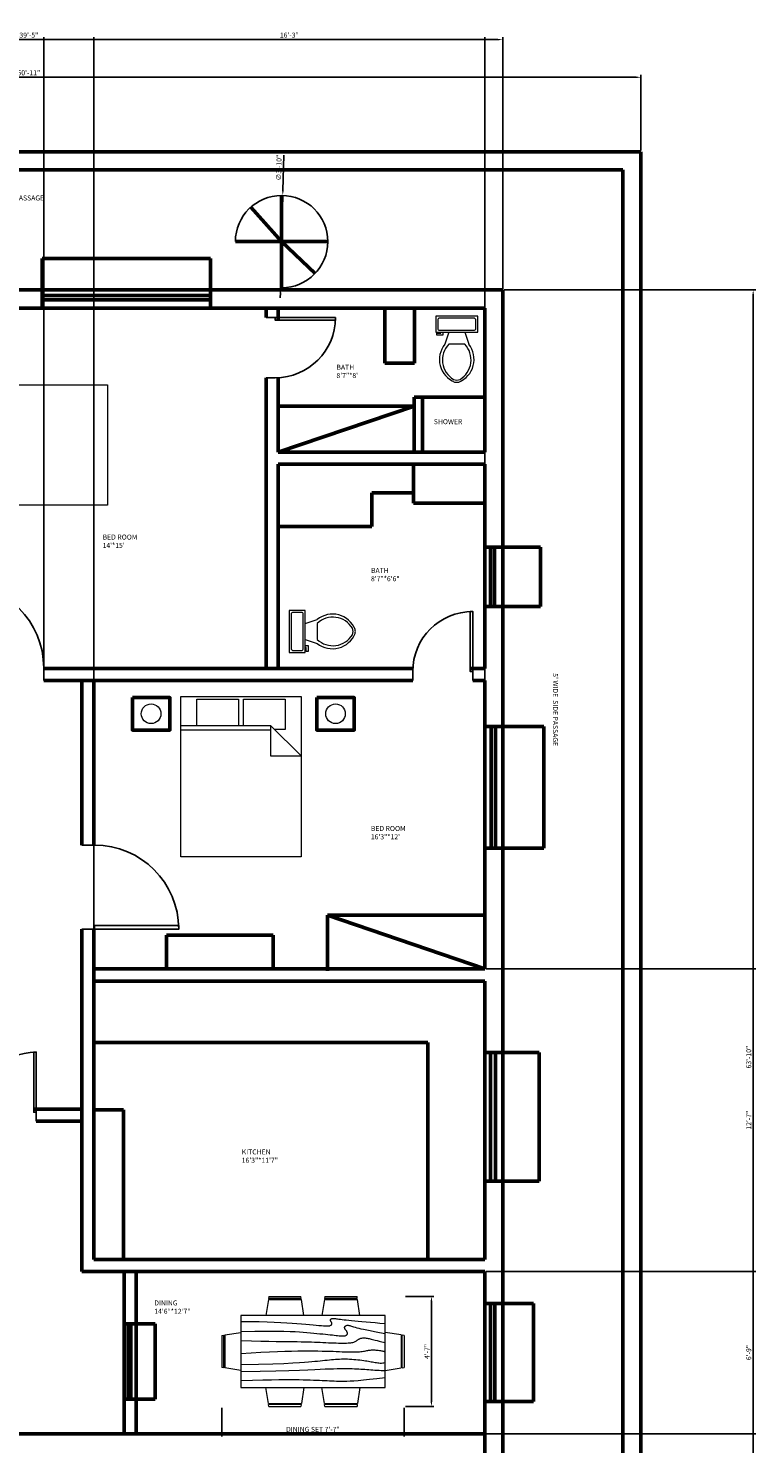
# Model space of a CAD drawing. Units: inches. Extents: x 5312 to 23584, y 2846 to 7447.
# Tile 11 of 12: x 11753 to 12116, y 3367 to 4074. Entities that reach past the tile are written whole.
import ezdxf

# ---------------------------------------------------------------- set-up
doc = ezdxf.new("R2010")
doc.units = ezdxf.units.IN
for name, color, linetype, lineweight in [('A-ANNO-DIMS', 2, 'Continuous', 18), ('A-ANNO-TEXT', 3, 'Continuous', 18), ('A-AREA-IDEN', 7, 'Continuous', 18), ('A-DOOR', 4, 'Continuous', 25), ('A-FLOR-FIXT', 9, 'Continuous', 18), ('A-FURN', 8, 'Continuous', 18), ('A-WALL', 7, 'Continuous', 50)]:
    doc.layers.add(name, color=color, linetype=linetype, lineweight=lineweight)
doc.styles.get("Standard").update_dxf_attribs({"font": 'arial.ttf'})
doc.dimstyles.new('ISO-25', dxfattribs={"dimtxt": 2.5, "dimasz": 2.5, "dimexe": 1.25, "dimexo": 0.625, "dimtad": 1, "dimlunit": 3, "dimtxsty": 'Standard', "dimcen": 2.5, "dimadec": 0, "dimazin": 0, "dimtfac": 1, "dimtmove": 0, "dimatfit": 3, "dimfxl": 1, "dimarcsym": 0})

# ---------------------------------------------------------------- blocks, each defined once
blk = doc.blocks.new('*U2')
for p, q in [((0, 0), (0, -6)), ((40, 0), (40, -6))]:
    blk.add_line(p, q)
blk.add_lwpolyline([(0, 0), (0, 40), (1.75, 40), (1.75, 0)], close=True)
blk.add_arc((0, 0), 40, 0, 90)
blk = doc.blocks.new('Toilet - top')
for p, q in [((9.5, -6), (9.5, -2)), ((-10, -8.5), (-8, -8.5)), ((-10, -9.5), (-10, -8.5)), ((-7, -9.5), (-10, -9.5)), ((-8, -8.5), (-8, -8)), ((-7, -8), (-7, -9.5)), ((-4, -8), (-6, -14)), ((4, -14), (-4, -14)), ((4, -8), (6, -14))]:
    blk.add_line(p, q)
blk.add_lwpolyline([(10.5, -8), (10.5, 0), (-10.5, 0), (-10.5, -8)], close=True)
for points in [[(-9.5, -2), (-9.5, -6)], [(8.5, -1), (-8.5, -1)], [(-8.5, -7), (8.5, -7)]]:
    blk.add_lwpolyline(points)
for centre, radius, start, end in [((-8.62, -1.88), 0.884, 81.8699, 188.1301), ((-8.62, -6.12), 0.884, 171.8699, 278.1301), ((8.62, -1.88), 0.884, 351.8699, 98.1301), ((8.62, -6.12), 0.884, 261.8699, 8.1301), ((3.52, -21.58), 12.17, 141.46911, 247.97143), ((4.2, -21.82), 11.33, 136.36773, 238.94682), ((-3.52, -21.58), 12.17, 292.02843, 38.53071), ((-4.2, -21.82), 11.33, 301.05301, 43.63209), ((0, -27.88), 4, 245.73182, 294.26817), ((0, -29), 4, 254.86053, 285.13947)]:
    blk.add_arc(centre, radius, start, end)
blk = doc.blocks.new('Bed - Queen')
for p, q in [((0, -80.00003), (0, 0)), ((0, 0), (59.99999, 0)), ((59.99999, 0), (59.99999, -80.00003)), ((7.99999, -1.2), (28.79998, -1.2)), ((7.99999, -14.4), (7.99999, -1.2)), ((28.79998, -1.2), (28.79998, -14.4)), ((31.19999, -1.2), (51.99999, -1.2)), ((31.19999, -14.4), (31.19999, -1.2)), ((51.99999, -1.2), (51.99999, -16.4)), ((0, -14.4), (44.8, -14.4)), ((44.8, -16.8), (0, -16.8)), ((59.99999, -29.6), (44.8, -14.4)), ((44.8, -14.4), (44.8, -29.6)), ((51.99999, -16.4), (46.79936, -16.4)), ((44.8, -29.6), (59.99999, -29.6)), ((59.99999, -80.00003), (0, -80.00003))]:
    blk.add_line(p, q)
blk = doc.blocks.new('Dining Set - 36 x 72 in.')
for p, q in [((-22.2343, 26.00059), (-23.4847, 17.99762)), ((-22.2304, 26), (-5.7608, 26)), ((-22, 27.5), (-22.1562, 26.50042)), ((-5.8416, 26.5), (-22.1534, 26.5)), ((-22, 27.5), (-6, 27.5)), ((-5.8437, 26.49966), (-6, 27.5)), ((-4.5152, 17.99762), (-5.7655, 25.99926)), ((5.7657, 26.00059), (4.5153, 17.99762)), ((5.7696, 26), (22.2392, 26)), ((6, 27.5), (5.8438, 26.50042)), ((22.1584, 26.5), (5.8466, 26.5)), ((6, 27.5), (22, 27.5)), ((22.1563, 26.49966), (22, 27.5)), ((23.4848, 17.99762), (22.2345, 25.99926)), ((36, 18), (-36, 18)), ((-36, 18), (-36, -18)), ((36, -18), (36, 18)), ((-45.5, 8), (-44.5004, 8.15617)), ((-45.5, 8), (-45.5, -8)), ((-44.5, -8.15843), (-44.5, 8.15338)), ((-44.0006, 8.23428), (-35.9976, 9.48474)), ((-44, 8.23041), (-44, -8.23915)), ((44.0006, 8.23428), (35.9976, 9.48474)), ((44, 8.23041), (44, -8.23915)), ((44.5, -8.15843), (44.5, 8.15338)), ((45.5, 8), (44.5005, 8.15617)), ((45.5, 8), (45.5, -8)), ((-44.4997, -8.15631), (-45.5, -8)), ((-35.9976, -9.48476), (-43.9993, -8.2345)), ((35.9976, -9.48476), (43.9993, -8.2345)), ((44.4997, -8.15631), (45.5, -8)), ((-36, -18), (36, -18)), ((-22.2343, -26.0006), (-23.4847, -17.99762)), ((-4.5152, -17.99762), (-5.7655, -25.99928)), ((5.7657, -26.0006), (4.5153, -17.99762)), ((23.4848, -17.99762), (22.2345, -25.99928)), ((-22.2304, -26), (-5.7608, -26)), ((-22, -27.5), (-22.1562, -26.50044)), ((-5.8416, -26.5), (-22.1534, -26.5)), ((-22, -27.5), (-6, -27.5)), ((-5.8437, -26.49967), (-6, -27.5)), ((5.7696, -26), (22.2392, -26)), ((6, -27.5), (5.8438, -26.50044)), ((22.1584, -26.5), (5.8466, -26.5)), ((6, -27.5), (22, -27.5)), ((22.1563, -26.49967), (22, -27.5))]:
    blk.add_line(p, q)
for points in [[(-36, 15), (-31.1772, 14.97754), (-26.8079, 14.91406), (-22.8538, 14.81543), (-19.276, 14.6875), (-16.0362, 14.53613), (-13.0957, 14.36718), (-10.4159, 14.18652), (-7.9583, 14), (-5.6904, 13.81315), (-3.6035, 13.63021), (-1.6954, 13.45508), (0.0365, 13.29166), (1.5945, 13.14388), (2.9811, 13.01562), (4.1988, 12.9108), (5.25, 12.83333), (6.1393, 12.78613), (6.8802, 12.76823), (7.4883, 12.77767), (7.9792, 12.8125), (8.3685, 12.87077), (8.6719, 12.95052), (8.9049, 13.0498), (9.0833, 13.16666), (9.2205, 13.29899), (9.3216, 13.44401), (9.3895, 13.59879), (9.4271, 13.76041), (9.4373, 13.92594), (9.4232, 14.09245), (9.3875, 14.257), (9.3333, 14.41666), (9.2638, 14.56917), (9.1836, 14.71484), (9.0975, 14.85465), (9.0104, 14.98958), (8.9272, 15.1206), (8.8529, 15.2487), (8.7922, 15.37483), (8.75, 15.5), (8.7305, 15.62467), (8.7344, 15.74739), (8.7617, 15.86621), (8.8125, 15.97916), (8.8867, 16.08431), (8.9844, 16.17968), (9.1055, 16.26334), (9.25, 16.33333), (9.4189, 16.38802), (9.6172, 16.42708), (9.8506, 16.45052), (10.125, 16.45833), (10.4463, 16.45052), (10.8203, 16.42708), (11.2529, 16.38802), (11.75, 16.33333), (12.3184, 16.26318), (12.9694, 16.17838), (13.7151, 16.07991), (14.5677, 15.96875), (15.5395, 15.84586), (16.6426, 15.71224), (17.8893, 15.56884), (19.2917, 15.41666), (20.859, 15.25667), (22.5879, 15.08984), (24.4721, 14.91715), (26.5052, 14.73958), (28.6809, 14.5581), (30.9929, 14.3737), (33.4347, 14.18733), (36, 14)], [(-36, 10), (-28.9766, 10.14274), (-23.1725, 10.20442), (-18.4241, 10.19775), (-14.5677, 10.13541), (-11.4399, 10.03011), (-8.877, 9.89453), (-6.7154, 9.74137), (-4.7917, 9.58333), (-2.9698, 9.43082), (-1.2246, 9.28515), (0.4415, 9.14534), (2.026, 9.01041), (3.5266, 8.87939), (4.9408, 8.7513), (6.266, 8.62516), (7.5, 8.5), (8.6411, 8.37549), (9.6914, 8.2539), (10.6538, 8.13818), (11.5312, 8.03125), (12.3267, 7.93603), (13.043, 7.85547), (13.6831, 7.79248), (14.25, 7.75), (14.7471, 7.7303), (15.1797, 7.73307), (15.5537, 7.75732), (15.875, 7.80208), (16.1494, 7.86637), (16.3828, 7.94922), (16.5811, 8.04964), (16.75, 8.16666), (16.8944, 8.29915), (17.0143, 8.44531), (17.1089, 8.60319), (17.1771, 8.77083), (17.218, 8.94629), (17.2305, 9.1276), (17.2137, 9.31282), (17.1667, 9.5), (17.0895, 9.6875), (16.987, 9.875), (16.8649, 10.0625), (16.7292, 10.25), (16.5856, 10.4375), (16.4401, 10.625), (16.2985, 10.8125), (16.1667, 11), (16.05, 11.18733), (15.9518, 11.3737), (15.8752, 11.5581), (15.8229, 11.73958), (15.798, 11.91715), (15.8034, 12.08984), (15.842, 12.25667), (15.9167, 12.41666), (16.0295, 12.56836), (16.1784, 12.70833), (16.3605, 12.83268), (16.5729, 12.9375), (16.8127, 13.01888), (17.0768, 13.07291), (17.3625, 13.0957), (17.6667, 13.08333), (17.9894, 13.03312), (18.3418, 12.94726), (18.7382, 12.82918), (19.1927, 12.68229), (19.7195, 12.51001), (20.3327, 12.31575), (21.0465, 12.10294), (21.875, 11.875), (22.8357, 11.63354), (23.959, 11.37304), (25.2786, 11.08618), (26.8282, 10.76562), (28.6414, 10.40405), (30.752, 9.99414), (33.1936, 9.52856), (36, 9)], [(-36, 5.5), (-30.7157, 5.3348), (-26.069, 5.20963), (-21.9946, 5.11767), (-18.4271, 5.05208), (-15.3009, 5.00602), (-12.5508, 4.97265), (-10.1112, 4.94515), (-7.9167, 4.91666), (-5.909, 4.88167), (-4.0586, 4.83984), (-2.3429, 4.79215), (-0.7396, 4.73958), (0.7739, 4.6831), (2.22, 4.6237), (3.6213, 4.56233), (5, 4.5), (6.373, 4.43782), (7.7344, 4.3776), (9.0723, 4.32129), (10.375, 4.27083), (11.6309, 4.22819), (12.8281, 4.19531), (13.9551, 4.17415), (15, 4.16666), (15.954, 4.17448), (16.819, 4.19791), (17.6001, 4.23698), (18.3021, 4.29166), (18.9299, 4.36198), (19.4883, 4.44791), (19.9823, 4.54948), (20.4167, 4.66666), (20.7969, 4.79899), (21.1302, 4.94401), (21.4245, 5.09879), (21.6875, 5.26041), (21.9271, 5.42594), (22.1511, 5.59245), (22.3672, 5.757), (22.5834, 5.91666), (22.8065, 6.06868), (23.0404, 6.21093), (23.2879, 6.34147), (23.5521, 6.45833), (23.8358, 6.55957), (24.142, 6.64323), (24.4735, 6.70735), (24.8334, 6.75), (25.2235, 6.76969), (25.642, 6.76692), (26.0858, 6.74267), (26.5521, 6.69791), (27.0379, 6.63362), (27.5404, 6.55078), (28.0565, 6.45036), (28.5834, 6.33333), (29.1242, 6.19987), (29.7071, 6.04687), (30.3661, 5.87044), (31.1354, 5.66666), (32.0493, 5.43164), (33.142, 5.16146), (34.4475, 4.85221), (36, 4.5)], [(-36, -1), (-30.7915, -0.6591), (-26.0195, -0.38216), (-21.6519, -0.16284), (-17.6563, 0.00521), (-14.0005, 0.12833), (-10.6523, 0.21289), (-7.5796, 0.26522), (-4.75, 0.29166), (-2.134, 0.29793), (0.2878, 0.28711), (2.5317, 0.26163), (4.6146, 0.22396), (6.5529, 0.17651), (8.3633, 0.12174), (10.0623, 0.06209), (11.6667, 0), (13.1899, -0.06201), (14.6341, -0.1211), (15.9982, -0.17432), (17.2813, -0.21875), (18.4823, -0.25147), (19.6003, -0.26953), (20.6343, -0.27002), (21.5834, -0.25), (22.4481, -0.20768), (23.2357, -0.14584), (23.9549, -0.06836), (24.6146, 0.02083), (25.2235, 0.11784), (25.7904, 0.21875), (26.3241, 0.31966), (26.8334, 0.41666), (27.3265, 0.50618), (27.8099, 0.58593), (28.2894, 0.65397), (28.7709, 0.70833), (29.2601, 0.74707), (29.763, 0.76823), (30.2855, 0.76985), (30.8334, 0.75), (31.4088, 0.70784), (31.9994, 0.64713), (32.589, 0.57275), (33.1615, 0.48958), (33.7008, 0.4025), (34.1908, 0.3164), (34.6153, 0.23616), (34.9584, 0.16666), (35.2099, 0.11165), (35.3848, 0.07031), (35.504, 0.04069), (35.5886, 0.02083), (35.6594, 0.00879), (35.7377, 0.0026), (35.8442, 0.00032), (36, 0)], [(-36, -6.5), (-27.1843, -6.31267), (-20.084, -6.1263), (-14.469, -5.9419), (-10.1094, -5.76042), (-6.7752, -5.58285), (-4.2363, -5.41016), (-2.2629, -5.24333), (-0.625, -5.08334), (0.8708, -4.93099), (2.2715, -4.78646), (3.5872, -4.64974), (4.8281, -4.52084), (6.0046, -4.39974), (7.127, -4.28646), (8.2053, -4.18099), (9.25, -4.08334), (10.2705, -3.99382), (11.2734, -3.91407), (12.2647, -3.84603), (13.25, -3.79167), (14.2354, -3.75293), (15.2266, -3.73177), (16.2295, -3.73015), (17.25, -3.75), (18.2912, -3.79248), (19.3451, -3.85547), (20.4009, -3.93604), (21.4479, -4.03125), (22.4754, -4.13819), (23.4727, -4.25391), (24.4289, -4.37549), (25.3334, -4.5), (26.1785, -4.62492), (26.9694, -4.74935), (27.7145, -4.87281), (28.4219, -4.99479), (29.1, -5.11483), (29.7572, -5.23242), (30.4016, -5.34709), (31.0417, -5.45834), (31.6837, -5.56437), (32.3262, -5.65821), (32.9658, -5.73153), (33.599, -5.77604), (34.2224, -5.78345), (34.8327, -5.74545), (35.4264, -5.65373), (36, -5.5)], [(-36, -10), (-26.4022, -9.81299), (-18.4675, -9.62891), (-11.9839, -9.45069), (-6.7396, -9.28125), (-2.5226, -9.12354), (0.8789, -8.98047), (3.6769, -8.85498), (6.0833, -8.75), (8.2767, -8.66765), (10.3021, -8.60677), (12.1712, -8.56543), (13.8958, -8.54167), (15.4876, -8.53353), (16.9583, -8.53907), (18.3197, -8.55632), (19.5834, -8.58334), (20.7616, -8.61841), (21.8685, -8.66081), (22.9188, -8.71004), (23.9271, -8.76563), (24.9081, -8.82707), (25.8763, -8.89388), (26.8465, -8.96558), (27.8334, -9.04167), (28.8474, -9.12118), (29.8828, -9.20117), (30.93, -9.27824), (31.9792, -9.34896), (33.0205, -9.40991), (34.0443, -9.45768), (35.0407, -9.48885), (36, -9.5)], [(-36, -14.5), (-30.0881, -14.33513), (-25.0332, -14.21224), (-20.7312, -14.12647), (-17.0781, -14.07292), (-13.97, -14.04671), (-11.3027, -14.04297), (-8.9724, -14.05681), (-6.875, -14.08334), (-4.9224, -14.11833), (-3.0905, -14.16016), (-1.3709, -14.20785), (0.2448, -14.26042), (1.7647, -14.3169), (3.1973, -14.3763), (4.5507, -14.43767), (5.8333, -14.5), (7.0554, -14.5621), (8.235, -14.62175), (9.3922, -14.67652), (10.5469, -14.72396), (11.7192, -14.76164), (12.929, -14.78711), (14.1965, -14.79794), (15.5417, -14.79167), (16.9933, -14.76424), (18.6152, -14.70508), (20.4804, -14.60197), (22.6615, -14.44271), (25.2312, -14.21509), (28.2624, -13.9069), (31.8277, -13.50594), (36, -13)]]:
    blk.add_lwpolyline(points)
blk = doc.blocks.new('*D19')
at = {"layer": 'A-ANNO-DIMS', "color": 0, "lineweight": -2, "transparency": 16777216}
for p, q in [((11447.29, 4012.53), (11447.29, 4050.35)), ((11449.79, 4049.1), (12055.79, 4049.1)), ((12058.29, 4012.53), (12058.29, 4050.35))]:
    blk.add_line(p, q, dxfattribs=at)
at = {"layer": 'A-ANNO-DIMS', "color": 0, "transparency": 16777216}
for points in [[(11449.79, 4049.52), (11449.79, 4048.69), (11447.29, 4049.1)], [(12055.79, 4049.52), (12055.79, 4048.69), (12058.29, 4049.1)]]:
    blk.add_solid(points, dxfattribs=at)
at = {"layer": 'DEFPOINTS', "color": 0, "transparency": 16777216}
for p in [(12058.29, 4049.1), (11447.29, 4011.91), (12058.29, 4011.91)]:
    blk.add_point(p, dxfattribs=at)
at = {"layer": 'A-ANNO-DIMS', "color": 0, "transparency": 16777216, "insert": (11752.79, 4051.01), "char_height": 2.5, "attachment_point": 5}
blk.add_mtext('50\'-11"', dxfattribs=at)
blk = doc.blocks.new('*D39')
at = {"layer": 'A-ANNO-DIMS', "color": 0, "lineweight": -2, "transparency": 16777216}
for p, q in [((11849.06, 3384.83), (11849.06, 3370.56)), ((11940.06, 3384.83), (11940.06, 3370.56)), ((11851.56, 3371.81), (11937.56, 3371.81))]:
    blk.add_line(p, q, dxfattribs=at)
at = {"layer": 'A-ANNO-DIMS', "color": 0, "transparency": 16777216}
for points in [[(11851.56, 3372.23), (11851.56, 3371.39), (11849.06, 3371.81)], [(11937.56, 3372.23), (11937.56, 3371.39), (11940.06, 3371.81)]]:
    blk.add_solid(points, dxfattribs=at)
at = {"layer": 'DEFPOINTS', "color": 0, "transparency": 16777216}
for p in [(11849.06, 3385.46), (11940.06, 3385.46), (11940.06, 3371.81)]:
    blk.add_point(p, dxfattribs=at)
at = {"layer": 'A-ANNO-DIMS', "color": 0, "transparency": 16777216, "insert": (11894.56, 3373.73), "char_height": 2.5, "attachment_point": 5}
blk.add_mtext('DINING SET 7\'-7"', dxfattribs=at)
blk = doc.blocks.new('*D40')
at = {"layer": 'A-ANNO-DIMS', "color": 0, "lineweight": -2, "transparency": 16777216}
for p, q in [((11940.69, 3440.46), (11954.96, 3440.46)), ((11953.71, 3387.96), (11953.71, 3437.96)), ((11940.69, 3385.46), (11954.96, 3385.46))]:
    blk.add_line(p, q, dxfattribs=at)
at = {"layer": 'A-ANNO-DIMS', "color": 0, "transparency": 16777216}
for points in [[(11953.3, 3437.96), (11954.13, 3437.96), (11953.71, 3440.46)], [(11953.3, 3387.96), (11954.13, 3387.96), (11953.71, 3385.46)]]:
    blk.add_solid(points, dxfattribs=at)
at = {"layer": 'DEFPOINTS', "color": 0, "transparency": 16777216}
for p in [(11940.06, 3440.46), (11953.71, 3440.46), (11940.06, 3385.46)]:
    blk.add_point(p, dxfattribs=at)
at = {"layer": 'A-ANNO-DIMS', "color": 0, "transparency": 16777216, "insert": (11951.84, 3412.96), "char_height": 2.5, "attachment_point": 5, "rotation": 90}
blk.add_mtext('4\'-7"', dxfattribs=at)
blk = doc.blocks.new('*D59')
at = {"layer": 'A-ANNO-DIMS', "color": 0, "lineweight": -2, "transparency": 16777216}
for p, q in [((11516.29, 3943.53), (11516.29, 4069.16)), ((11518.79, 4067.91), (11986.79, 4067.91)), ((11989.29, 3943.53), (11989.29, 4069.16))]:
    blk.add_line(p, q, dxfattribs=at)
at = {"layer": 'A-ANNO-DIMS', "color": 0, "transparency": 16777216}
for points in [[(11518.79, 4068.32), (11518.79, 4067.49), (11516.29, 4067.91)], [(11986.79, 4068.32), (11986.79, 4067.49), (11989.29, 4067.91)]]:
    blk.add_solid(points, dxfattribs=at)
at = {"layer": 'DEFPOINTS', "color": 0, "transparency": 16777216}
for p in [(11989.29, 4067.91), (11516.29, 3942.91), (11989.29, 3942.91)]:
    blk.add_point(p, dxfattribs=at)
at = {"layer": 'A-ANNO-DIMS', "color": 0, "transparency": 16777216, "insert": (11752.79, 4069.81), "char_height": 2.5, "attachment_point": 5}
blk.add_mtext('39\'-5"', dxfattribs=at)
blk = doc.blocks.new('*D60')
at = {"layer": 'A-ANNO-DIMS', "color": 0, "lineweight": -2, "transparency": 16777216}
for p, q in [((11989.92, 3942.91), (12115.54, 3942.91)), ((12114.29, 3940.41), (12114.29, 3179.41)), ((11989.92, 3176.91), (12115.54, 3176.91))]:
    blk.add_line(p, q, dxfattribs=at)
at = {"layer": 'A-ANNO-DIMS', "color": 0, "transparency": 16777216}
for points in [[(12113.87, 3940.41), (12114.71, 3940.41), (12114.29, 3942.91)], [(12113.87, 3179.41), (12114.71, 3179.41), (12114.29, 3176.91)]]:
    blk.add_solid(points, dxfattribs=at)
at = {"layer": 'DEFPOINTS', "color": 0, "transparency": 16777216}
for p in [(11989.29, 3942.91), (11989.29, 3176.91), (12114.29, 3176.91)]:
    blk.add_point(p, dxfattribs=at)
at = {"layer": 'A-ANNO-DIMS', "color": 0, "transparency": 16777216, "insert": (12112.39, 3559.91), "char_height": 2.5, "attachment_point": 5, "rotation": 90}
blk.add_mtext('63\'-10"', dxfattribs=at)
blk = doc.blocks.new('*D62')
at = {"layer": 'A-ANNO-DIMS', "color": 0, "lineweight": -2, "transparency": 16777216}
for p, q in [((11785.29, 3604.53), (11785.29, 4069.16)), ((11787.79, 4067.91), (11977.79, 4067.91)), ((11980.29, 3604.53), (11980.29, 4069.16))]:
    blk.add_line(p, q, dxfattribs=at)
at = {"layer": 'A-ANNO-DIMS', "color": 0, "transparency": 16777216}
for points in [[(11787.79, 4068.32), (11787.79, 4067.49), (11785.29, 4067.91)], [(11977.79, 4068.32), (11977.79, 4067.49), (11980.29, 4067.91)]]:
    blk.add_solid(points, dxfattribs=at)
at = {"layer": 'DEFPOINTS', "color": 0, "transparency": 16777216}
for p in [(11980.29, 4067.91), (11785.29, 3603.91), (11980.29, 3603.91)]:
    blk.add_point(p, dxfattribs=at)
at = {"layer": 'A-ANNO-DIMS', "color": 0, "transparency": 16777216, "insert": (11882.79, 4069.81), "char_height": 2.5, "attachment_point": 5}
blk.add_mtext('16\'-3"', dxfattribs=at)
blk = doc.blocks.new('*D63')
at = {"layer": 'A-ANNO-DIMS', "color": 0, "lineweight": -2, "transparency": 16777216}
for p, q in [((11980.92, 3603.91), (12115.54, 3603.91)), ((12114.29, 3601.41), (12114.29, 3455.41)), ((11980.92, 3452.91), (12115.54, 3452.91))]:
    blk.add_line(p, q, dxfattribs=at)
at = {"layer": 'A-ANNO-DIMS', "color": 0, "transparency": 16777216}
for points in [[(12113.87, 3601.41), (12114.71, 3601.41), (12114.29, 3603.91)], [(12113.87, 3455.41), (12114.71, 3455.41), (12114.29, 3452.91)]]:
    blk.add_solid(points, dxfattribs=at)
at = {"layer": 'DEFPOINTS', "color": 0, "transparency": 16777216}
for p in [(11980.29, 3603.91), (11980.29, 3452.91), (12114.29, 3452.91)]:
    blk.add_point(p, dxfattribs=at)
at = {"layer": 'A-ANNO-DIMS', "color": 0, "transparency": 16777216, "insert": (12112.41, 3528.41), "char_height": 2.5, "attachment_point": 5, "rotation": 90}
blk.add_mtext('12\'-7"', dxfattribs=at)
blk = doc.blocks.new('*D64')
at = {"layer": 'A-ANNO-DIMS', "color": 0, "lineweight": -2, "transparency": 16777216}
for p, q in [((11980.92, 3452.91), (12115.54, 3452.91)), ((12114.29, 3450.41), (12114.29, 3374.41)), ((11980.92, 3371.91), (12115.54, 3371.91))]:
    blk.add_line(p, q, dxfattribs=at)
at = {"layer": 'A-ANNO-DIMS', "color": 0, "transparency": 16777216}
for points in [[(12113.87, 3450.41), (12114.71, 3450.41), (12114.29, 3452.91)], [(12113.87, 3374.41), (12114.71, 3374.41), (12114.29, 3371.91)]]:
    blk.add_solid(points, dxfattribs=at)
at = {"layer": 'DEFPOINTS', "color": 0, "transparency": 16777216}
for p in [(11980.29, 3452.91), (11980.29, 3371.91), (12114.29, 3371.91)]:
    blk.add_point(p, dxfattribs=at)
at = {"layer": 'A-ANNO-DIMS', "color": 0, "transparency": 16777216, "insert": (12112.39, 3412.41), "char_height": 2.5, "attachment_point": 5, "rotation": 90}
blk.add_mtext('6\'-9"', dxfattribs=at)
blk = doc.blocks.new('*D70')
at = {"layer": 'A-ANNO-DIMS', "color": 0, "lineweight": -2, "transparency": 16777216}
for p, q in [((11719.53, 3753.53), (11719.53, 4069.16)), ((11722.03, 4067.91), (11757.73, 4067.91)), ((11760.23, 3752.99), (11760.23, 4069.16))]:
    blk.add_line(p, q, dxfattribs=at)
at = {"layer": 'A-ANNO-DIMS', "color": 0, "transparency": 16777216}
for points in [[(11722.03, 4068.32), (11722.03, 4067.49), (11719.53, 4067.91)], [(11757.73, 4068.32), (11757.73, 4067.49), (11760.23, 4067.91)]]:
    blk.add_solid(points, dxfattribs=at)
at = {"layer": 'DEFPOINTS', "color": 0, "transparency": 16777216}
for p in [(11760.23, 4067.91), (11719.53, 3752.91), (11760.23, 3752.37)]:
    blk.add_point(p, dxfattribs=at)
at = {"layer": 'A-ANNO-DIMS', "color": 0, "transparency": 16777216, "insert": (11739.88, 4069.83), "char_height": 2.5, "attachment_point": 5}
blk.add_mtext('3\'-4 1/2"', dxfattribs=at)
blk = doc.blocks.new('*D99')
at = {"layer": 'A-ANNO-DIMS', "color": 0, "lineweight": -2, "transparency": 16777216}
for p, q in [((11879.99, 4010.21), (11879.56, 3992.6)), ((11878.39, 3943.99), (11879.5, 3990.1)), ((11878.33, 3941.49), (11878.27, 3938.99))]:
    blk.add_line(p, q, dxfattribs=at)
at = {"layer": 'A-ANNO-DIMS', "color": 0, "transparency": 16777216}
for points in [[(11879.15, 3992.61), (11879.98, 3992.59), (11879.5, 3990.1)], [(11877.91, 3941.5), (11878.75, 3941.48), (11878.39, 3943.99)]]:
    blk.add_solid(points, dxfattribs=at)
at = {"layer": 'DEFPOINTS', "color": 0, "transparency": 16777216}
for p in [(11879.5, 3990.1), (11878.39, 3943.99)]:
    blk.add_point(p, dxfattribs=at)
at = {"layer": 'A-ANNO-DIMS', "color": 0, "transparency": 16777216, "insert": (11877.87, 4003.98), "char_height": 2.5, "attachment_point": 5, "rotation": 88.6184}
blk.add_mtext('∅3\'-10"', dxfattribs=at)

msp = doc.modelspace()

# ---------------------------------------------------------------- linework, layer by layer
at = {"layer": 'A-DOOR'}
msp.add_arc((11878.946, 3967.047), 23.062, 270, 180, dxfattribs=at)
at = {"layer": 'A-FURN'}
for centre in [(11813.81, 3731.316), (11905.84, 3731.316)]:
    msp.add_circle(centre, 4.897, dxfattribs=at)
at = {"layer": 'A-WALL'}
for p, q in [((11447.292, 4011.907), (12058.292, 4011.907)), ((12049.292, 4011.907), (12047.292, 4011.907)), ((12058.292, 4011.907), (12058.292, 2931.907)), ((11456.292, 4002.907), (12049.292, 4002.907)), ((12049.292, 4002.907), (12049.292, 2940.907)), ((11878.946, 3990.109), (11878.946, 3943.985)), ((11878.946, 3967.047), (11863.587, 3984.25)), ((11855.884, 3967.047), (11902.009, 3967.047)), ((11878.946, 3967.047), (11895.633, 3951.128)), ((11759.506, 3933.907), (11759.506, 3958.699)), ((11759.506, 3958.699), (11843.506, 3958.699)), ((11843.506, 3958.699), (11843.506, 3933.907)), ((11516.292, 3942.907), (11989.292, 3942.907)), ((11759.506, 3940.141), (11843.506, 3940.141)), ((11759.506, 3937.919), (11843.506, 3937.919)), ((11989.292, 3942.907), (11989.292, 3176.907)), ((11703.292, 3933.907), (11980.292, 3933.907)), ((11871.292, 3933.907), (11871.292, 3929.115)), ((11877.292, 3933.907), (11877.292, 3927.803)), ((11930.424, 3933.907), (11930.424, 3906.377)), ((11945.223, 3906.377), (11945.223, 3933.907)), ((11980.292, 3933.907), (11980.292, 3861.907)), ((11930.424, 3906.377), (11945.223, 3906.377)), ((11871.292, 3899.115), (11871.292, 3753.907)), ((11877.292, 3899.153), (11877.292, 3861.907)), ((11945.099, 3861.907), (11945.099, 3889.48)), ((11945.099, 3889.48), (11980.292, 3889.48)), ((11949.202, 3889.48), (11949.202, 3861.907)), ((11945.099, 3884.959), (11877.292, 3884.959)), ((11877.292, 3861.907), (11945.099, 3884.959)), ((11877.292, 3861.907), (11980.292, 3861.907)), ((11877.292, 3855.907), (11980.292, 3855.907)), ((11877.292, 3855.907), (11877.292, 3753.907)), ((11944.718, 3855.907), (11944.718, 3836.553)), ((11980.292, 3855.907), (11980.292, 3753.907)), ((11924.035, 3824.815), (11924.035, 3841.57)), ((11924.035, 3841.57), (11944.718, 3841.57)), ((11944.718, 3836.553), (11980.292, 3836.553)), ((11877.292, 3824.815), (11924.035, 3824.815)), ((11980.292, 3814.572), (12008.224, 3814.572)), ((11983.187, 3814.572), (11983.187, 3784.921)), ((11985.15, 3814.572), (11985.15, 3784.921)), ((12008.224, 3814.572), (12008.224, 3784.921)), ((12008.224, 3784.921), (11980.292, 3784.921)), ((11760.226, 3753.907), (11944.405, 3753.907)), ((11973.055, 3753.907), (11980.292, 3753.907)), ((11760.226, 3747.907), (11944.367, 3747.907)), ((11779.292, 3747.907), (11779.292, 3665.76)), ((11785.292, 3747.907), (11785.292, 3665.76)), ((11974.367, 3747.907), (11980.292, 3747.907)), ((11980.292, 3747.907), (11980.292, 3603.907)), ((11980.292, 3725.018), (11989.292, 3725.018)), ((11983.519, 3725.018), (11983.519, 3664.264)), ((11985.612, 3725.018), (11985.612, 3664.264)), ((12009.812, 3725.018), (11989.292, 3725.018)), ((12009.812, 3664.264), (12009.812, 3725.018)), ((11980.292, 3664.264), (12009.812, 3664.264)), ((11901.803, 3602.993), (11901.803, 3630.775)), ((11901.803, 3630.775), (11980.292, 3630.775)), ((11901.803, 3630.775), (11980.292, 3603.907)), ((11779.292, 3623.76), (11779.292, 3452.907)), ((11785.292, 3623.76), (11785.292, 3458.907)), ((11821.56, 3603.907), (11821.56, 3620.869)), ((11821.56, 3620.869), (11874.669, 3620.869)), ((11874.669, 3620.869), (11874.669, 3603.907)), ((11785.292, 3603.907), (11980.292, 3603.907)), ((11785.292, 3597.907), (11980.292, 3597.907)), ((11980.292, 3597.907), (11980.292, 3458.907)), ((11785.292, 3567.251), (11951.963, 3567.251)), ((11951.963, 3567.251), (11951.963, 3458.907)), ((11980.292, 3562.19), (11989.292, 3562.19)), ((11983.224, 3562.19), (11983.224, 3497.994)), ((11985.678, 3562.19), (11985.678, 3497.994)), ((11989.292, 3562.19), (12007.508, 3562.19)), ((12007.508, 3562.19), (12007.508, 3497.994)), ((11755.205, 3533.907), (11779.292, 3533.907)), ((11785.292, 3533.517), (11800.037, 3533.517)), ((11800.037, 3533.517), (11800.037, 3458.907)), ((11756.517, 3527.907), (11779.292, 3527.907)), ((11980.292, 3497.994), (11989.292, 3497.994)), ((12007.508, 3497.994), (11989.292, 3497.994)), ((11785.292, 3458.907), (11980.292, 3458.907)), ((11779.292, 3452.907), (11980.292, 3452.907)), ((11800.292, 3452.907), (11800.292, 3371.907)), ((11806.292, 3452.907), (11806.292, 3371.907)), ((11980.292, 3452.907), (11980.292, 3185.907)), ((11980.292, 3436.857), (11989.292, 3436.857)), ((11983.215, 3436.857), (11983.215, 3388.021)), ((11985.381, 3436.857), (11985.381, 3388.021)), ((11989.292, 3436.857), (12004.694, 3436.857)), ((12004.694, 3436.857), (12004.694, 3388.545)), ((11806.292, 3426.806), (11800.292, 3426.806)), ((11802.308, 3426.806), (11802.308, 3389.181)), ((11803.688, 3426.806), (11803.688, 3389.181)), ((11806.292, 3426.806), (11815.84, 3426.806)), ((11815.84, 3426.806), (11815.84, 3389.181)), ((11806.292, 3389.181), (11800.292, 3389.181)), ((11815.84, 3389.181), (11806.292, 3389.181)), ((11980.292, 3388.021), (11989.292, 3388.021)), ((11989.292, 3388.021), (12004.694, 3388.021)), ((12004.694, 3388.021), (12004.694, 3388.545)), ((11571.113, 3371.907), (11980.292, 3371.907))]:
    msp.add_line(p, q, dxfattribs=at)
for points in [[(11804.462, 3739.424), (11823.158, 3739.424), (11823.158, 3723.207), (11804.462, 3723.207)], [(11896.492, 3739.424), (11915.188, 3739.424), (11915.188, 3723.207), (11896.492, 3723.207)]]:
    msp.add_lwpolyline(points, close=True, dxfattribs=at)

# ---------------------------------------------------------------- block references
at = {"layer": 'A-DOOR', "rotation": 270}
for p, xscale, yscale, zscale in [((11875.792, 3929.115), 0.75, 0.75, 0.75), ((11785.592, 3623.76), -1.049999999999999, 1.049999999999999, 1.049999999999999)]:
    msp.add_blockref('*U2', p, dxfattribs=dict(at, xscale=xscale, yscale=yscale, zscale=zscale))
at = {"layer": 'A-DOOR'}
for p, xscale, yscale, zscale in [((11718.226, 3754.207), 1.049999999999999, 1.049999999999999, 1.049999999999999), ((11974.367, 3752.407), -0.75, 0.75, 0.75), ((11756.517, 3532.407), -0.75, 0.75, 0.75)]:
    msp.add_blockref('*U2', p, dxfattribs=dict(at, xscale=xscale, yscale=yscale, zscale=zscale))
at = {"layer": 'A-FLOR-FIXT'}
msp.add_blockref('Toilet - top', (11966.344, 3929.804), dxfattribs=at)
at = {"layer": 'A-FLOR-FIXT', "rotation": 89.99999999999999}
msp.add_blockref('Toilet - top', (11882.739, 3772.446), dxfattribs=at)
at = {"layer": 'A-FURN', "rotation": 90}
msp.add_blockref('Bed - Queen', (11712.054, 3835.548), dxfattribs=at)
at = {"layer": 'A-FURN'}
for name, p in [('Bed - Queen', (11828.66, 3739.87)), ('Dining Set - 36 x 72 in.', (11894.565, 3412.959))]:
    msp.add_blockref(name, p, dxfattribs=at)

# ---------------------------------------------------------------- texts
at = {"layer": 'A-ANNO-TEXT', "char_height": 2.5, "attachment_point": 1}
for s, width, insert in [("5' WIDE REAR PASSAGE", 78.67751, (11723.753, 3990.095)), ('SHOWER', 17.19091, (11954.909, 3878.41))]:
    msp.add_mtext_dynamic_manual_height_columns(s, width=width, gutter_width=12.5, heights=[0], dxfattribs=dict(at, insert=insert))
at = {"layer": 'A-ANNO-TEXT', "insert": (12016.86, 3751.57), "char_height": 2.5, "attachment_point": 1, "rotation": 270}
msp.add_mtext_dynamic_manual_height_columns("5' WIDE  SIDE PASSAGE", width=42.12812, gutter_width=12.5, heights=[0], dxfattribs=at)
at = {"layer": 'A-AREA-IDEN', "char_height": 2.5, "attachment_point": 1}
for s, width, insert in [('BATH\\P8\'7"*8\'', 15.46736, (11906.304, 3905.609)), ("BED ROOM\\P14'*15'", 56.00673, (11789.592, 3820.797)), ('BATH\\P8\'7"*6\'6"', 35.97251, (11923.555, 3804.157)), ('BED ROOM\\P16\'3"*12\'', 49.90282, (11923.47, 3675.307)), ('KITCHEN\\P16\'3"*11\'7"', 105.00049, (11859.039, 3513.836)), ('DINING\\P14\'6"*12\'7"', 34.15837, (11815.378, 3438.426))]:
    msp.add_mtext_dynamic_manual_height_columns(s, width=width, gutter_width=12.5, heights=[0], dxfattribs=dict(at, insert=insert))

# ---------------------------------------------------------------- dimensions: what is measured, and where the dimension line sits
at = {"layer": 'A-ANNO-DIMS'}
for base, p1, p2, override, picture, middle in [((11989.292, 4067.907), (11516.292, 3942.907), (11989.292, 3942.907), {"dimdec": 1, "dimlfac": 1, "dimrnd": 0, "dimzin": 1, "dimdsep": 46, "dimlunit": 4, "dimfrac": 2}, '*D59', (11752.792, 4069.809)), ((11760.226, 4067.907), (11719.526, 3752.908), (11760.226, 3752.37), {"dimdec": 1, "dimlfac": 1, "dimrnd": 0, "dimzin": 1, "dimdsep": 46, "dimlunit": 4, "dimfrac": 2}, '*D70', (11739.876, 4069.826)), ((11980.292, 4067.907), (11785.292, 3603.907), (11980.292, 3603.907), {"dimdec": 1, "dimlfac": 1, "dimrnd": 0, "dimzin": 1, "dimdsep": 46, "dimlunit": 4, "dimfrac": 2}, '*D62', (11882.792, 4069.809)), ((12058.292, 4049.105), (11447.292, 4011.907), (12058.292, 4011.907), {"dimclrd": 0, "dimclre": 0, "dimclrt": 0}, '*D19', (11752.792, 4051.006))]:
    dim = msp.add_linear_dim(base=base, p1=p1, p2=p2, dimstyle='ISO-25', override=override, dxfattribs=at)
    dim.commit()
    dim.dimension.update_dxf_attribs({"geometry": picture, "text_midpoint": middle})
dim = msp.add_diameter_dim_2p(p1=(11878.39, 3943.991), p2=(11879.502, 3990.103), dimstyle='ISO-25', override={"dimdec": 1, "dimlfac": 1, "dimrnd": 0, "dimzin": 1, "dimdsep": 46, "dimlunit": 4, "dimfrac": 2}, dxfattribs=at)
dim.commit()
dim.dimension.update_dxf_attribs({"geometry": '*D99', "text_midpoint": (11879.836, 4003.936), "dimtype": 163})
for base, p1, p2, override, picture, middle in [((12114.292, 3176.907), (11989.292, 3942.907), (11989.292, 3176.907), {"dimdec": 1, "dimlfac": 1, "dimrnd": 0, "dimzin": 1, "dimdsep": 46, "dimlunit": 4, "dimfrac": 2}, '*D60', (12112.389, 3559.907)), ((12114.292, 3452.907), (11980.292, 3603.907), (11980.292, 3452.907), {"dimdec": 1, "dimlfac": 1, "dimrnd": 0, "dimzin": 1, "dimdsep": 46, "dimlunit": 4, "dimfrac": 2}, '*D63', (12112.411, 3528.407)), ((12114.292, 3371.907), (11980.292, 3452.907), (11980.292, 3371.907), {"dimdec": 1, "dimlfac": 1, "dimrnd": 0, "dimzin": 1, "dimdsep": 46, "dimlunit": 4, "dimfrac": 2}, '*D64', (12112.39, 3412.407)), ((11953.715, 3440.459), (11940.065, 3385.459), (11940.065, 3440.459), {"dimdec": 1, "dimrnd": 0, "dimzin": 1, "dimlunit": 4, "dimfrac": 2}, '*D40', (11951.84, 3412.959))]:
    dim = msp.add_linear_dim(base=base, p1=p1, p2=p2, angle=90, dimstyle='ISO-25', override=override, dxfattribs=at)
    dim.commit()
    dim.dimension.update_dxf_attribs({"geometry": picture, "text_midpoint": middle})
dim = msp.add_linear_dim(base=(11940.065, 3371.809), p1=(11849.065, 3385.459), p2=(11940.065, 3385.459), text='DINING SET <>', dimstyle='ISO-25', override={"dimdec": 1, "dimrnd": 0, "dimzin": 1, "dimlunit": 4, "dimfrac": 2}, dxfattribs=at)
dim.commit()
dim.dimension.update_dxf_attribs({"geometry": '*D39', "text_midpoint": (11894.565, 3373.727)})

doc.saveas('drawing.dxf')
